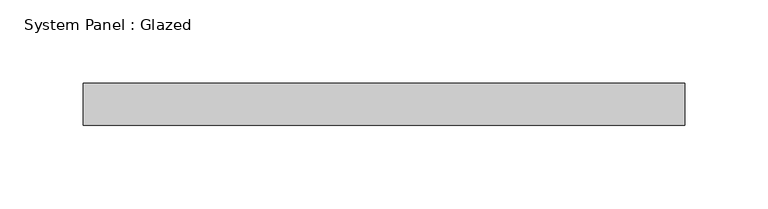
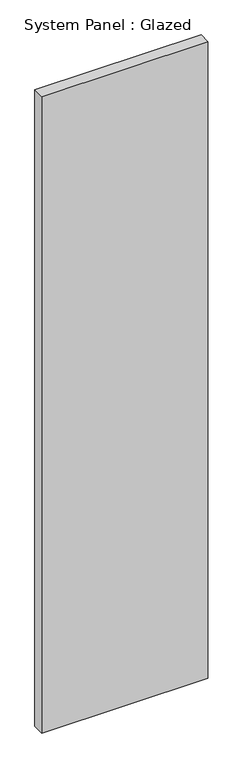
"""IFC4 building model written with IfcOpenShell, lengths in millimetres: plate geometry, System Panel : Glazed."""

from ifc_helpers import new_model, si_unit, origin, origin_with_axes, place, context, project, spatial, polyline, outline, extrude, source, transform, mapped, element, save


def system_panel_glazed_c2792dd2(model_context):
    return source(origin(), model_context, "Body", "SweptSolid", [
        extrude(outline(polyline([(180.975, 19.05), (-180.975, 19.05), (-180.975, 44.45), (180.975, 44.45), (180.975, 19.05)])), origin_with_axes(), (0.0, 0.0, 1.0), 1466.034917),
    ])


if __name__ == "__main__":
    model = new_model("IFC4")
    model_context = context("Model", 3, world=origin())
    ifc_project = project(units=[si_unit("LENGTHUNIT", "METRE", prefix="MILLI")], contexts=[model_context])
    site = spatial("IfcSite", under=ifc_project)
    building = spatial("IfcBuilding", under=site)
    placement = place(None, origin())
    system_panel_glazed_shape = system_panel_glazed_c2792dd2(model_context)
    element("IfcPlate", 1, ObjectType="System Panel : Glazed", at=placement, inside=building, context=model_context, shape_type="MappedRepresentation", body=[
        mapped(system_panel_glazed_shape, transform((0.0, 0.0, 0.0), x_axis=(1.0, 0.0, 0.0), y_axis=(0.0, 1.0, 0.0), z_axis=(0.0, 0.0, 1.0))),
    ])
    save(model, "model.ifc")

# Revit data of these elements
# Type "System Panel : Glazed"
#   Construction Type Id = "GSP4R"
#   Analytic Construction = "1/8 in Pilkington single glazing"
#   Visual Light Transmittance = 0.9
#   Solar Heat Gain Coefficient = 0.86
#   Heat Transfer Coefficient (U) = 1.18115 BTU/(h·ft²·°F)
#   Define Thermal Properties by = 1
# Element 1 (IfcPlate, "System Panel : Glazed")
#   Materials on its faces: "Glass"
# Materials
#   "Glass": class "Glass", colour RGB 0 128 192, transparency 0.75, Description = "Soda Lime Glass", Cost = 0
